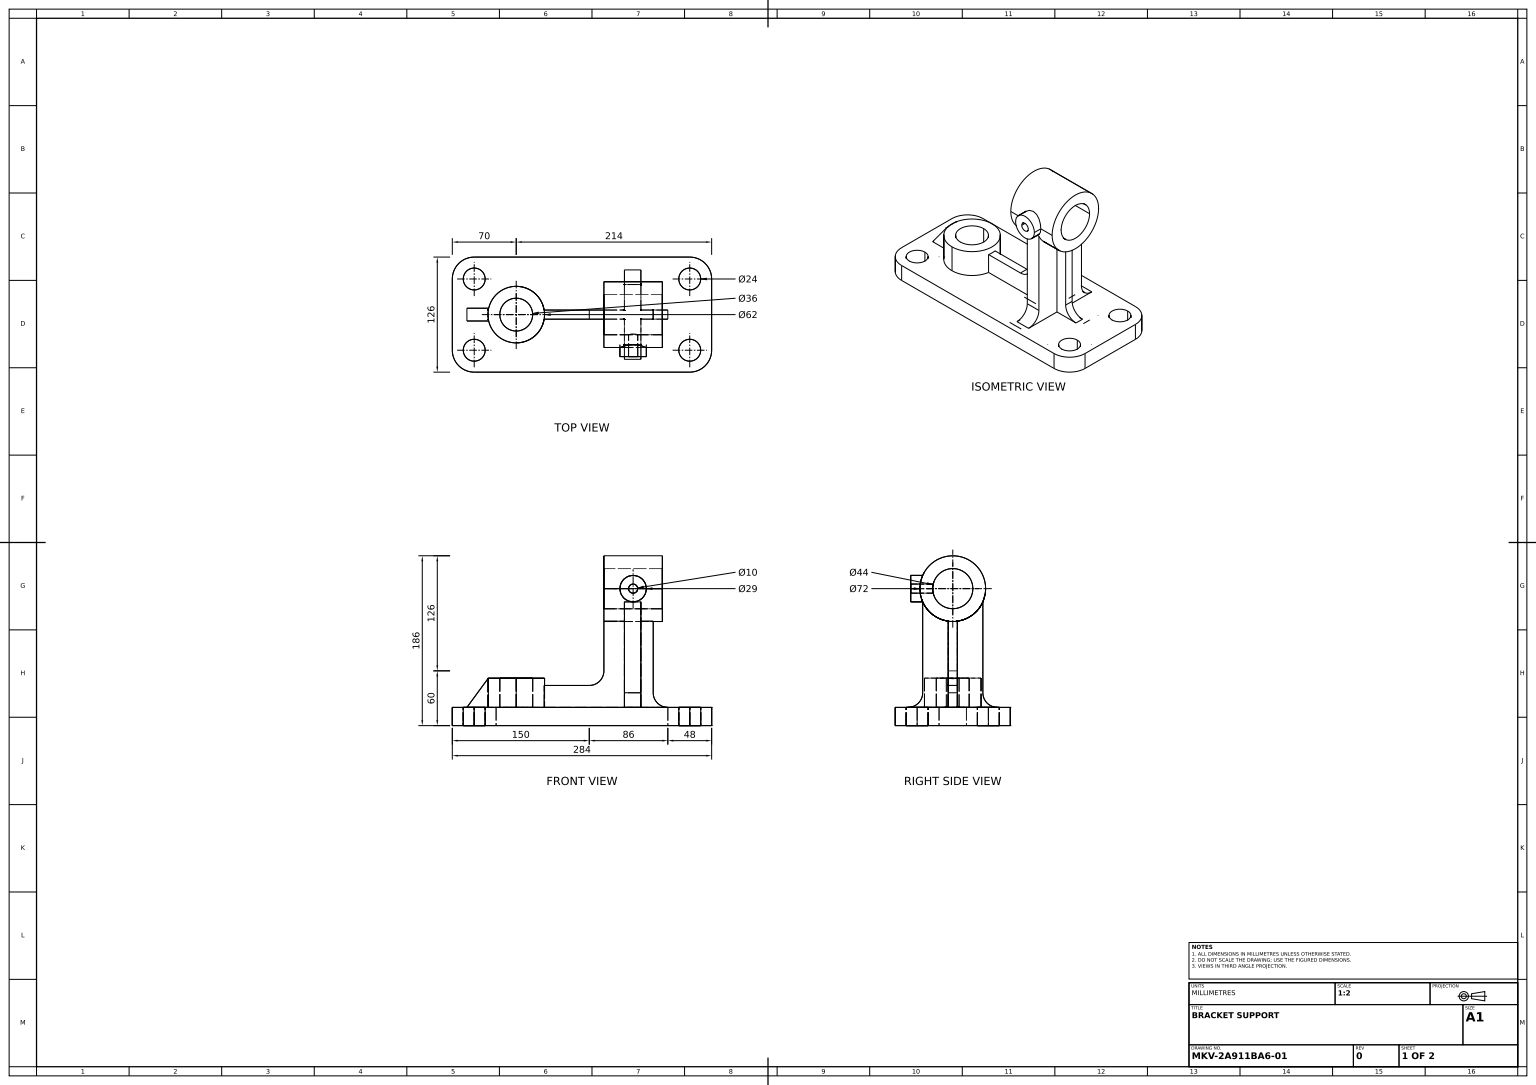
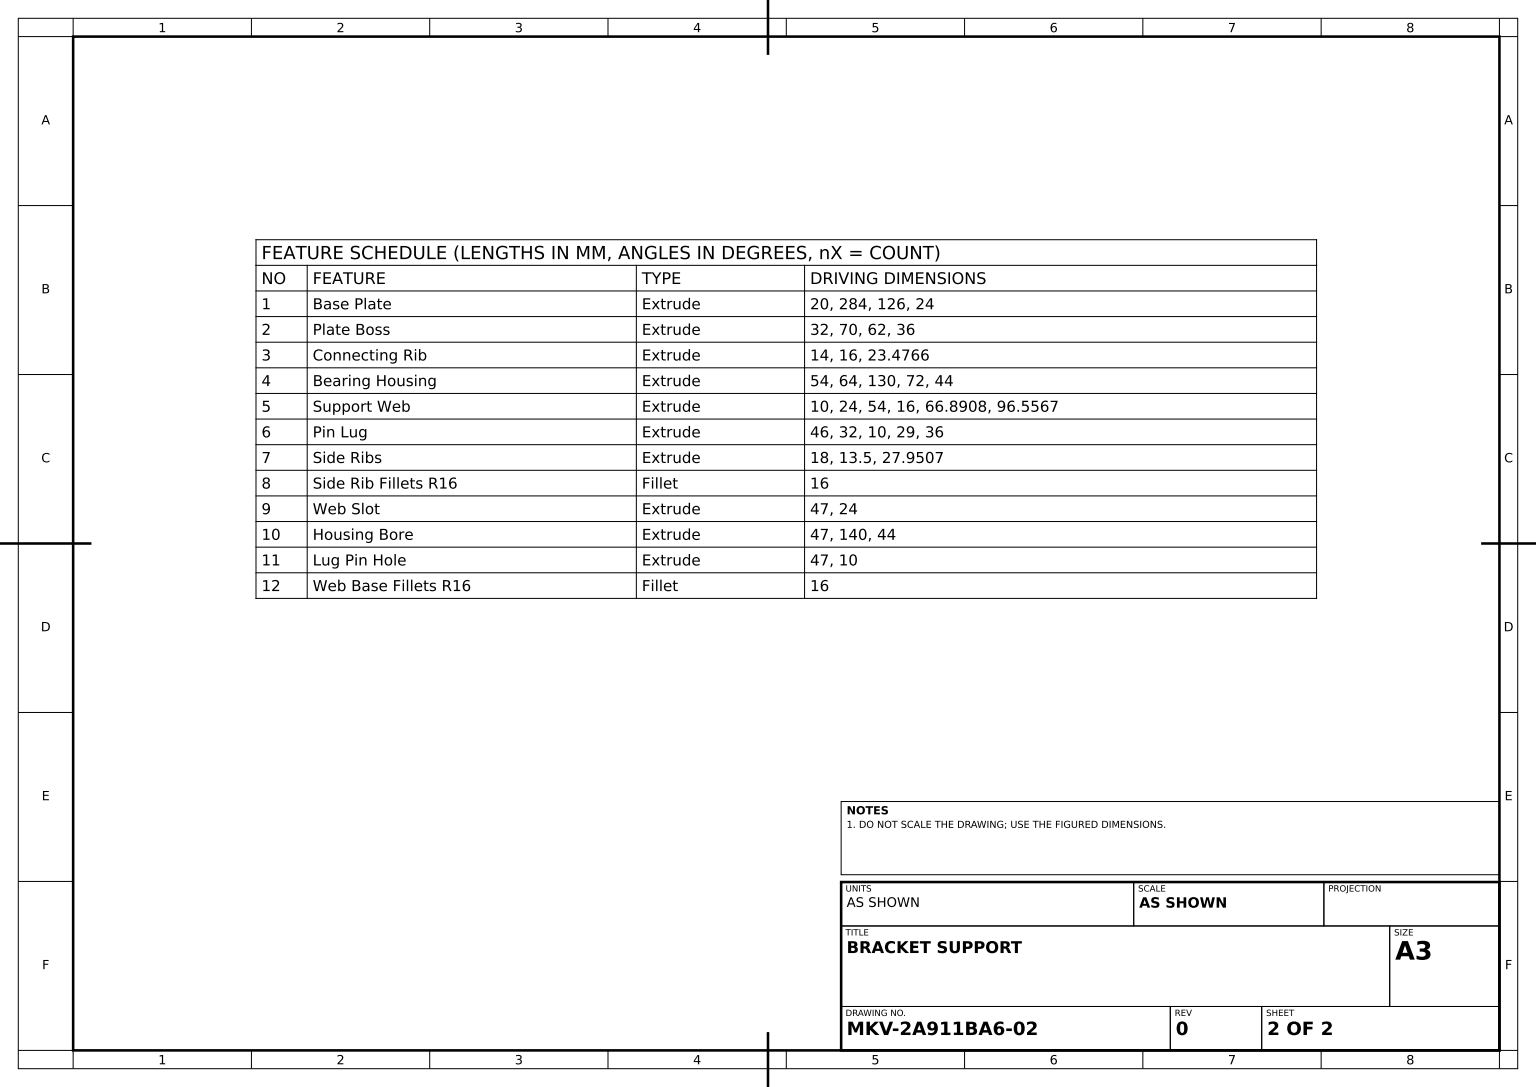
SolidWorks part; units mm, degrees
material "Plain Carbon Steel"
ref_plane "Front Plane" through (0, 0, 0) normal (0, 0, 1) x (1, 0, 0)
ref_plane "Top Plane" through (0, 0, 0) normal (0, 1, 0) x (1, 0, 0)
ref_plane "Right Plane" through (0, 0, 0) normal (1, 0, 0) x (0, 0, -1)
sketch "Base Plate Sketch" plane through (0, 0, 0) normal (0, 1, 0) x (1, 0, 0)
  line L1 (-118, 63) -> (118, 63)
  line L2 (-142, 39) -> (-142, -39)
  line L3 (-118, -63) -> (118, -63)
  line L4 (142, 39) -> (142, -39)
  line L5 (-142, 63) -> (142, -63) construction
  line L6 (-142, -63) -> (142, 63) construction
  arc A0 (-118, 63) -> (-142, 39) centre (-118, 39) ccw
  arc A1 (-142, -39) -> (-118, -63) centre (-118, -39) ccw
  arc A2 (118, -63) -> (142, -39) centre (118, -39) ccw
  arc A3 (118, 63) -> (142, 39) centre (118, 39) cw
  point P0 (0, 0)
  dimension "D3" = 24
  dimension "D1" = 284
  dimension "D2" = 126
extrude "Base Plate" add sketch "Base Plate Sketch" along normal mid plane 20
sketch "Plate Boss Sketch" plane through (0, 10, 0) normal (0, 1, 0) x (1, 0, 0)
  line L0 (-142, 39) -> (-142, -39) construction
  circle A0 centre (-72, 0) radius 18
  circle A1 centre (-72, 0) radius 31
  dimension "D2" = 62
  dimension "D3" = 36
  dimension "D1" = 70
extrude "Plate Boss" add sketch "Plate Boss Sketch" along normal blind 32
sketch "Connecting Rib Sketch" plane through (0, 0, 0) normal (0, 0, 1) x (1, 0, 0)
  line L1 (-118, 10) -> (118, 10) construction
  line L4 (-126, 10) -> (-102.5234, 42)
  line L5 (-142, 10) -> (-142, -10) construction
  line L6 (-126, 10) -> (-102.5234, 10)
  line L8 (-102.5234, 10) -> (-102.5234, 42)
  line L9 (-41, 42) -> (-103, 42) construction
  dimension "D1" = 16
  dimension "D2" = 23.4766
extrude "Connecting Rib" add sketch "Connecting Rib Sketch" along normal mid plane 14 contours L4 L8 L6
ref_plane "Plane1" through (88, 0, 0) normal (1, 0, 0) x (0, 0, -1)
sketch "Bearing Housing Sketch" plane through (88, 0, 0) normal (1, 0, 0) x (0, 0, -1)
  line L0 (-39, 10) -> (39, 10) construction
  circle A0 centre (0, 140) radius 36
  circle A1 centre (0, 140) radius 22
  dimension "D2" = 72
  dimension "D3" = 44
  dimension "D1" = 130
extrude "Bearing Housing" add sketch "Bearing Housing Sketch" against normal blind 64 separate body
sketch "Support Web Sketch" plane through (0, 0, 0) normal (0, 0, 1) x (1, 0, 0)
  line L0 (-42.8908, 10) -> (-42.8908, 34)
  line L1 (-42.8908, 34) -> (8, 34)
  line L2 (24, 50) -> (24, 106.5567)
  line L3 (-42.8908, 10) -> (78, 10)
  line L4 (-118, 10) -> (118, 10) construction
  line L5 (78, 10) -> (78, 106.5567)
  line L6 (78, 106.5567) -> (24, 106.5567)
  line L7 (24, 176) -> (24, 104) construction
  arc A0 (8, 34) -> (24, 50) centre (8, 50) ccw
  dimension "D3" = 16
  dimension "D1" = 24
  dimension "D2" = 54
  dimension "D4" = 54
  dimension "D5" = 66.8908
  dimension "D6" = 96.5567
extrude "Support Web" add sketch "Support Web Sketch" along normal mid plane 10 contours L1 A0 L2 L6 L5 L3 L0
sketch "Pin Lug Sketch" plane through (0, 0, 0) normal (0, 0, 1) x (1, 0, 0)
  line L0 (24, 176) -> (24, 104.3489) construction
  line L1 (88, 176) -> (24, 176) construction
  circle A0 centre (56, 140) radius 5
  circle A1 centre (56, 140) radius 14.5
  dimension "D2" = 10
  dimension "D3" = 29
  dimension "D1" = 32
  dimension "D4" = 36
extrude "Pin Lug" add sketch "Pin Lug Sketch" along normal blind 46
sketch "Side Ribs Sketch" plane through (78, 0, 0) normal (1, 0, 0) x (0, 0, -1)
  line L0 (-32.9507, 125.5) -> (-32.9507, 10)
  line L1 (-39, 10) -> (39, 10) construction
  line L3 (32.9507, 125.5) -> (32.9507, 10)
  line L4 (32.9507, 10) -> (-32.9507, 10)
  line L5 (5, 10) -> (5, 104.3489) construction
  arc A0 (-32.9507, 154.5) -> (-32.9507, 125.5) centre (0, 140) ccw construction
  circle A1 centre (0, 140) radius 36 construction
  arc A2 (-32.9507, 125.5) -> (32.9507, 125.5) centre (0, 140) ccw
  dimension "D1" = 27.9507
extrude "Side Ribs" add sketch "Side Ribs Sketch" against normal blind 18 from offset 13.5 offset against normal yes
fillet "Side Rib Fillets R16" radius 16 2 edges at (55.5, 10, -32.9507) (55.5, 10, 32.9507)
sketch "Web Slot Sketch" plane through (0, 10, 0) normal (0, 1, 0) x (1, 0, 0)
  circle A0 centre (-118, 39) radius 12
  circle A1 centre (-118, -39) radius 12
  circle A2 centre (118, -39) radius 12
  circle A3 centre (118, 39) radius 12
  arc A4 (-118, 63) -> (-142, 39) centre (-118, 39) ccw construction
  arc A5 (-142, -39) -> (-118, -63) centre (-118, -39) ccw construction
  arc A6 (118, -63) -> (142, -39) centre (118, -39) ccw construction
  arc A7 (142, 39) -> (118, 63) centre (118, 39) ccw construction
  dimension "D1" = 24
extrude "Web Slot" cut sketch "Web Slot Sketch" against normal blind 47
sketch "Housing Bore Sketch" plane through (88, 0, 0) normal (1, 0, 0) x (0, 0, -1)
  circle A0 centre (0, 140) radius 22
  dimension "D2" = 44
  dimension "D1" = 140
extrude "Housing Bore" cut sketch "Housing Bore Sketch" against normal blind 47
sketch "Lug Pin Hole Sketch" plane through (0, 0, 46) normal (0, 0, 1) x (1, 0, 0)
  circle A0 centre (56, 140) radius 5
  dimension "D1" = 10
extrude "Lug Pin Hole" cut sketch "Lug Pin Hole Sketch" against normal blind 47
fillet "Web Base Fillets R16" radius 16 1 edges at (78, 10, 0)
